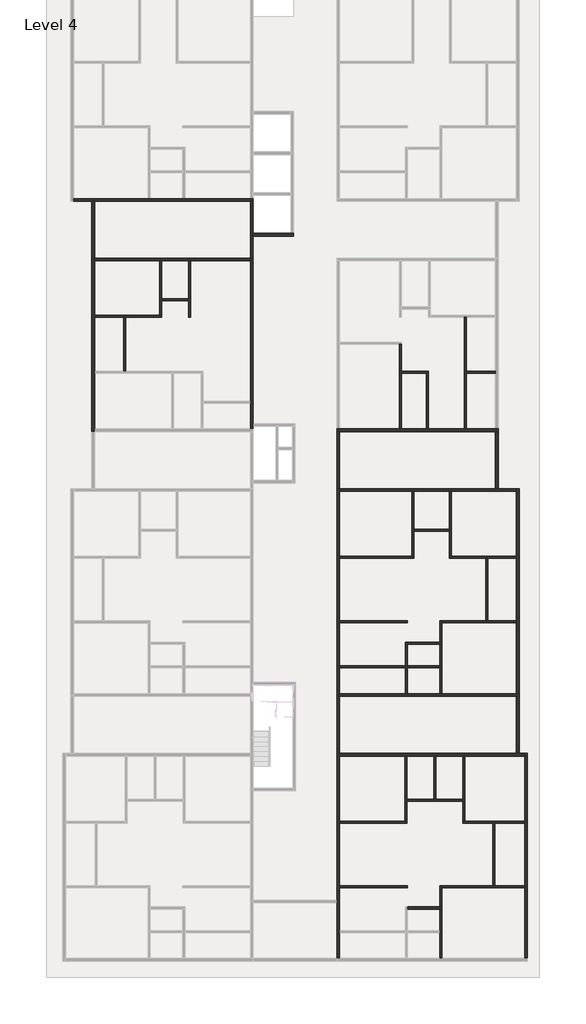
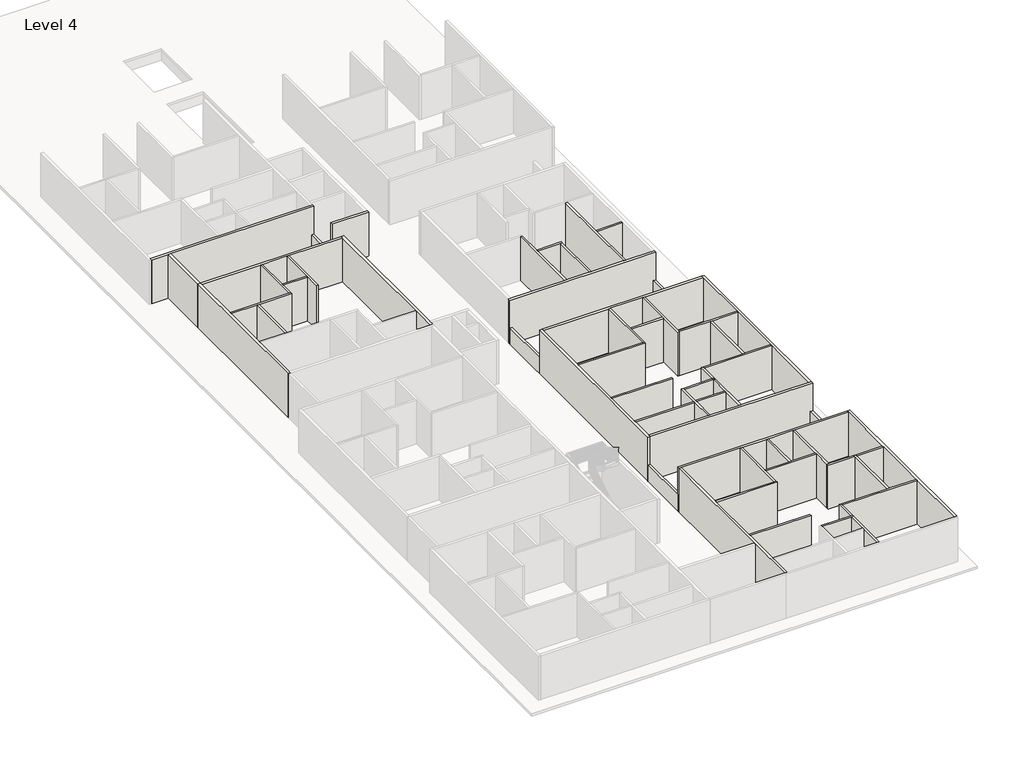
# One storey, part 2 of 8: 56 walls.
"""IFC4 building model written with IfcOpenShell, lengths in millimetres."""

from ifc_helpers import new_model, si_unit, frame, origin, place, context, project, spatial, polyline, outline, extrude, faceted_brep, element, save

model = new_model("IFC4")

# Units and contexts
model_context = context("Model", 3, world=origin())
ifc_project = project(units=[si_unit("LENGTHUNIT", "METRE", prefix="MILLI")], contexts=[model_context])

# Site, building, storey
site = spatial("IfcSite", under=ifc_project)
building = spatial("IfcBuilding", under=site)
storey = spatial("IfcBuildingStorey", under=building, Name="Level 4", Elevation=34378.6172466)

# Walls
placement = place(None, origin())
element("IfcWall", 1, ObjectType="4.5\"", at=placement, inside=storey, context=model_context, shape_type="Brep", body=[
    faceted_brep([(-12531.5544854, 2100.0216096, 34378.6172466), (-10907.2415084, 2100.0216096, 34378.6172466), (-10792.9415084, 2100.0216096, 34378.6172466), (-8759.6544854, 2100.0216096, 34378.6172466), (-8759.6544854, 2100.0216096, 37426.6172466), (-10792.9415084, 2100.0216096, 37426.6172466), (-10907.2415084, 2100.0216096, 37426.6172466), (-12531.5544854, 2100.0216096, 37426.6172466), (-12531.5544854, 2214.3216096, 34378.6172466), (-12531.5544854, 2214.3216096, 37426.6172466), (-8873.9544854, 2214.3216096, 37426.6172466), (-8759.6544854, 2214.3216096, 37426.6172466), (-8759.6544854, 2214.3216096, 34378.6172466), (-8873.9544854, 2214.3216096, 34378.6172466)], [[[0, 1, 2, 3, 4, 5, 6, 7]], [[8, 9, 10, 11, 12, 13]], [[3, 2, 1, 0, 8, 13, 12]], [[0, 7, 9, 8]], [[4, 3, 12, 11]], [[7, 6, 5, 4, 11, 10, 9]]]),
])
element("IfcWall", 2, ObjectType="4.5\"", at=placement, inside=storey, context=model_context, shape_type="Brep", body=[
    faceted_brep([(-8759.6544854, 2214.3216096, 34378.6172466), (-8759.6544854, 3014.4216096, 34378.6172466), (-8759.6544854, 3128.7216096, 34378.6172466), (-8759.6544854, 5264.2743917, 34378.6172466), (-8759.6544854, 5264.2743917, 37426.6172466), (-8759.6544854, 3128.7216096, 37426.6172466), (-8759.6544854, 3014.4216096, 37426.6172466), (-8759.6544854, 2214.3216096, 37426.6172466), (-8873.9544854, 2214.3216096, 34378.6172466), (-8873.9544854, 2214.3216096, 37426.6172466), (-8873.9544854, 5264.2743917, 37426.6172466), (-8873.9544854, 5264.2743917, 34378.6172466)], [[[0, 1, 2, 3, 4, 5, 6, 7]], [[8, 9, 10, 11]], [[3, 2, 1, 0, 8, 11]], [[0, 7, 9, 8]], [[4, 3, 11, 10]], [[7, 6, 5, 4, 10, 9]]]),
])
element("IfcWall", 3, ObjectType="4.5\"", at=placement, inside=storey, context=model_context, shape_type="Brep", body=[
    faceted_brep([(-7235.6544854, 5264.2743917, 34378.6172466), (-7235.6544854, 3128.7216096, 34378.6172466), (-7235.6544854, 3014.4216096, 34378.6172466), (-7235.6544854, 2100.0216096, 34378.6172466), (-7235.6544854, 2100.0216096, 37426.6172466), (-7235.6544854, 3014.4216096, 37426.6172466), (-7235.6544854, 3128.7216096, 37426.6172466), (-7235.6544854, 5264.2743917, 37426.6172466), (-7121.3544854, 5264.2743917, 34378.6172466), (-7121.3544854, 5264.2743917, 37426.6172466), (-7121.3544854, 2100.0216096, 37426.6172466), (-7121.3544854, 2100.0216096, 34378.6172466)], [[[0, 1, 2, 3, 4, 5, 6, 7]], [[8, 9, 10, 11]], [[3, 2, 1, 0, 8, 11]], [[4, 3, 11, 10]], [[0, 7, 9, 8]], [[7, 6, 5, 4, 10, 9]]]),
])
element("IfcWall", 4, ObjectType="4.5\"", at=placement, inside=storey, context=model_context, shape_type="SweptSolid", body=[
    extrude(outline(polyline([(-7235.6544854, 3014.4216096), (-8759.6544854, 3014.4216096), (-8759.6544854, 3128.7216096), (-7235.6544854, 3128.7216096), (-7235.6544854, 3014.4216096)])), frame((0.0, 0.0, 34378.6172466), z_axis=(0.0, 0.0, 1.0), x_axis=(1.0, 0.0, 0.0)), (0.0, 0.0, 1.0), 3048.0),
])
element("IfcWall", 5, ObjectType="4.5\"", at=placement, inside=storey, context=model_context, shape_type="SweptSolid", body=[
    extrude(outline(polyline([(-10907.2415084, -947.4344126), (-10907.2415084, 2100.0216096), (-10792.9415084, 2100.0216096), (-10792.9415084, -947.4344126), (-10907.2415084, -947.4344126)])), frame((0.0, 0.0, 34378.6172466), z_axis=(0.0, 0.0, 1.0), x_axis=(1.0, 0.0, 0.0)), (0.0, 0.0, 1.0), 3048.0),
])
element("IfcWall", 6, ObjectType="4.5\"", at=placement, inside=storey, context=model_context, shape_type="Brep", body=[
    faceted_brep([(5056.6584916, -31173.4344126, 34378.6172466), (6885.4584916, -31173.4344126, 34378.6172466), (6999.7584916, -31173.4344126, 34378.6172466), (6999.7584916, -31173.4344126, 37426.6172466), (6885.4584916, -31173.4344126, 37426.6172466), (5056.6584916, -31173.4344126, 37426.6172466), (5056.6584916, -31059.1344126, 34378.6172466), (5056.6584916, -31059.1344126, 37426.6172466), (6885.4584916, -31059.1344126, 37426.6172466), (6999.7584916, -31059.1344126, 37426.6172466), (6999.7584916, -31059.1344126, 34378.6172466), (6885.4584916, -31059.1344126, 34378.6172466)], [[[0, 1, 2, 3, 4, 5]], [[6, 7, 8, 9, 10, 11]], [[2, 1, 0, 6, 11, 10]], [[0, 5, 7, 6]], [[3, 2, 10, 9]], [[5, 4, 3, 9, 8, 7]]]),
])
element("IfcWall", 7, ObjectType="4.5\"", at=placement, inside=storey, context=model_context, shape_type="Brep", body=[
    faceted_brep([(6885.4584916, -31173.4344126, 34378.6172466), (6885.4584916, -32392.6344126, 34378.6172466), (6885.4584916, -32506.9344126, 34378.6172466), (6885.4584916, -33954.7344126, 34378.6172466), (6885.4584916, -33954.7344126, 37426.6172466), (6885.4584916, -32506.9344126, 37426.6172466), (6885.4584916, -32392.6344126, 37426.6172466), (6885.4584916, -31173.4344126, 37426.6172466), (6999.7584916, -31173.4344126, 34378.6172466), (6999.7584916, -31173.4344126, 37426.6172466), (6999.7584916, -33954.7344126, 37426.6172466), (6999.7584916, -33954.7344126, 34378.6172466)], [[[0, 1, 2, 3, 4, 5, 6, 7]], [[8, 9, 10, 11]], [[3, 2, 1, 0, 8, 11]], [[0, 7, 9, 8]], [[4, 3, 11, 10]], [[7, 6, 5, 4, 10, 9]]]),
])
element("IfcWall", 8, ObjectType="4.5\"", at=placement, inside=storey, context=model_context, shape_type="Brep", body=[
    faceted_brep([(6999.7584916, -31059.1344126, 34378.6172466), (6999.7584916, -29966.9344126, 34378.6172466), (6999.7584916, -29852.6344126, 34378.6172466), (6999.7584916, -29852.6344126, 37426.6172466), (6999.7584916, -29966.9344126, 37426.6172466), (6999.7584916, -31059.1344126, 37426.6172466), (6885.4584916, -31059.1344126, 34378.6172466), (6885.4584916, -31059.1344126, 37426.6172466), (6885.4584916, -29852.6344126, 37426.6172466), (6885.4584916, -29852.6344126, 34378.6172466)], [[[0, 1, 2, 3, 4, 5]], [[6, 7, 8, 9]], [[2, 1, 0, 6, 9]], [[0, 5, 7, 6]], [[3, 2, 9, 8]], [[5, 4, 3, 8, 7]]]),
])
element("IfcWall", 9, ObjectType="4.5\"", at=placement, inside=storey, context=model_context, shape_type="Brep", body=[
    faceted_brep([(6999.7584916, -29966.9344126, 34378.6172466), (11660.6584916, -29966.9344126, 34378.6172466), (11660.6584916, -29966.9344126, 37426.6172466), (6999.7584916, -29966.9344126, 37426.6172466), (6999.7584916, -29852.6344126, 34378.6172466), (6999.7584916, -29852.6344126, 37426.6172466), (9869.9584916, -29852.6344126, 37426.6172466), (9984.2584916, -29852.6344126, 37426.6172466), (11660.6584916, -29852.6344126, 37426.6172466), (11660.6584916, -29852.6344126, 34378.6172466), (9984.2584916, -29852.6344126, 34378.6172466), (9869.9584916, -29852.6344126, 34378.6172466)], [[[0, 1, 2, 3]], [[4, 5, 6, 7, 8, 9, 10, 11]], [[1, 0, 4, 11, 10, 9]], [[0, 3, 5, 4]], [[2, 1, 9, 8]], [[3, 2, 8, 7, 6, 5]]]),
])
element("IfcWall", 10, ObjectType="4.5\"", at=placement, inside=storey, context=model_context, shape_type="SweptSolid", body=[
    extrude(outline(polyline([(5056.6584916, -29966.9344126), (1259.3584916, -29966.9344126), (1259.3584916, -29852.6344126), (5056.6584916, -29852.6344126), (5056.6584916, -29966.9344126)])), frame((0.0, 0.0, 34378.6172466), z_axis=(0.0, 0.0, 1.0), x_axis=(1.0, 0.0, 0.0)), (0.0, 0.0, 1.0), 3048.0),
])
element("IfcWall", 11, ObjectType="4.5\"", at=placement, inside=storey, context=model_context, shape_type="Brep", body=[
    faceted_brep([(1259.3584916, -26347.4344126, 34378.6172466), (5031.2584916, -26347.4344126, 34378.6172466), (5031.2584916, -26347.4344126, 37426.6172466), (1259.3584916, -26347.4344126, 37426.6172466), (1259.3584916, -26233.1344126, 34378.6172466), (1259.3584916, -26233.1344126, 37426.6172466), (4916.9584916, -26233.1344126, 37426.6172466), (5031.2584916, -26233.1344126, 37426.6172466), (5031.2584916, -26233.1344126, 34378.6172466), (4916.9584916, -26233.1344126, 34378.6172466)], [[[0, 1, 2, 3]], [[4, 5, 6, 7, 8, 9]], [[1, 0, 4, 9, 8]], [[0, 3, 5, 4]], [[2, 1, 8, 7]], [[3, 2, 7, 6, 5]]]),
])
element("IfcWall", 12, ObjectType="4.5\"", at=placement, inside=storey, context=model_context, shape_type="Brep", body=[
    faceted_brep([(5031.2584916, -26233.1344126, 34378.6172466), (5031.2584916, -25128.2344126, 34378.6172466), (5031.2584916, -25013.9344126, 34378.6172466), (5031.2584916, -22575.5344126, 34378.6172466), (5031.2584916, -22575.5344126, 37426.6172466), (5031.2584916, -25013.9344126, 37426.6172466), (5031.2584916, -25128.2344126, 37426.6172466), (5031.2584916, -26233.1344126, 37426.6172466), (4916.9584916, -26233.1344126, 34378.6172466), (4916.9584916, -26233.1344126, 37426.6172466), (4916.9584916, -22575.5344126, 37426.6172466), (4916.9584916, -22575.5344126, 34378.6172466)], [[[0, 1, 2, 3, 4, 5, 6, 7]], [[8, 9, 10, 11]], [[3, 2, 1, 0, 8, 11]], [[0, 7, 9, 8]], [[4, 3, 11, 10]], [[7, 6, 5, 4, 10, 9]]]),
])
element("IfcWall", 13, ObjectType="4.5\"", at=placement, inside=storey, context=model_context, shape_type="Brep", body=[
    faceted_brep([(9984.2584916, -29852.6344126, 34378.6172466), (9984.2584916, -26347.4344126, 34378.6172466), (9984.2584916, -26233.1344126, 34378.6172466), (9984.2584916, -26233.1344126, 37426.6172466), (9984.2584916, -26347.4344126, 37426.6172466), (9984.2584916, -29852.6344126, 37426.6172466), (9869.9584916, -29852.6344126, 34378.6172466), (9869.9584916, -29852.6344126, 37426.6172466), (9869.9584916, -26347.4344126, 37426.6172466), (9869.9584916, -26233.1344126, 37426.6172466), (9869.9584916, -26233.1344126, 34378.6172466), (9869.9584916, -26347.4344126, 34378.6172466)], [[[0, 1, 2, 3, 4, 5]], [[6, 7, 8, 9, 10, 11]], [[2, 1, 0, 6, 11, 10]], [[0, 5, 7, 6]], [[3, 2, 10, 9]], [[5, 4, 3, 9, 8, 7]]]),
])
element("IfcWall", 14, ObjectType="4.5\"", at=placement, inside=storey, context=model_context, shape_type="SweptSolid", body=[
    extrude(outline(polyline([(11660.6584916, -26347.4344126), (9984.2584916, -26347.4344126), (9984.2584916, -26233.1344126), (11660.6584916, -26233.1344126), (11660.6584916, -26347.4344126)])), frame((0.0, 0.0, 34378.6172466), z_axis=(0.0, 0.0, 1.0), x_axis=(1.0, 0.0, 0.0)), (0.0, 0.0, 1.0), 3048.0),
])
element("IfcWall", 15, ObjectType="4.5\"", at=placement, inside=storey, context=model_context, shape_type="Brep", body=[
    faceted_brep([(9869.9584916, -26233.1344126, 34378.6172466), (8307.8584916, -26233.1344126, 34378.6172466), (8193.5584916, -26233.1344126, 34378.6172466), (8193.5584916, -26233.1344126, 37426.6172466), (8307.8584916, -26233.1344126, 37426.6172466), (9869.9584916, -26233.1344126, 37426.6172466), (9869.9584916, -26347.4344126, 34378.6172466), (9869.9584916, -26347.4344126, 37426.6172466), (8193.5584916, -26347.4344126, 37426.6172466), (8193.5584916, -26347.4344126, 34378.6172466)], [[[0, 1, 2, 3, 4, 5]], [[6, 7, 8, 9]], [[2, 1, 0, 6, 9]], [[0, 5, 7, 6]], [[3, 2, 9, 8]], [[5, 4, 3, 8, 7]]]),
])
element("IfcWall", 16, ObjectType="4.5\"", at=placement, inside=storey, context=model_context, shape_type="Brep", body=[
    faceted_brep([(8307.8584916, -26233.1344126, 34378.6172466), (8307.8584916, -22575.5344126, 34378.6172466), (8307.8584916, -22575.5344126, 37426.6172466), (8307.8584916, -26233.1344126, 37426.6172466), (8193.5584916, -26233.1344126, 34378.6172466), (8193.5584916, -26233.1344126, 37426.6172466), (8193.5584916, -25128.2344126, 37426.6172466), (8193.5584916, -25013.9344126, 37426.6172466), (8193.5584916, -22575.5344126, 37426.6172466), (8193.5584916, -22575.5344126, 34378.6172466), (8193.5584916, -25013.9344126, 34378.6172466), (8193.5584916, -25128.2344126, 34378.6172466)], [[[0, 1, 2, 3]], [[4, 5, 6, 7, 8, 9, 10, 11]], [[1, 0, 4, 11, 10, 9]], [[0, 3, 5, 4]], [[2, 1, 9, 8]], [[3, 2, 8, 7, 6, 5]]]),
])
element("IfcWall", 17, ObjectType="4.5\"", at=placement, inside=storey, context=model_context, shape_type="Brep", body=[
    faceted_brep([(5031.2584916, -25128.2344126, 34378.6172466), (8193.5584916, -25128.2344126, 34378.6172466), (8193.5584916, -25128.2344126, 37426.6172466), (5031.2584916, -25128.2344126, 37426.6172466), (5031.2584916, -25013.9344126, 34378.6172466), (5031.2584916, -25013.9344126, 37426.6172466), (6555.2584916, -25013.9344126, 37426.6172466), (6669.5584916, -25013.9344126, 37426.6172466), (8193.5584916, -25013.9344126, 37426.6172466), (8193.5584916, -25013.9344126, 34378.6172466), (6669.5584916, -25013.9344126, 34378.6172466), (6555.2584916, -25013.9344126, 34378.6172466)], [[[0, 1, 2, 3]], [[4, 5, 6, 7, 8, 9, 10, 11]], [[1, 0, 4, 11, 10, 9]], [[0, 3, 5, 4]], [[2, 1, 9, 8]], [[3, 2, 8, 7, 6, 5]]]),
])
element("IfcWall", 18, ObjectType="4.5\"", at=placement, inside=storey, context=model_context, shape_type="SweptSolid", body=[
    extrude(outline(polyline([(6555.2584916, -25013.9344126), (6555.2584916, -22575.5344126), (6669.5584916, -22575.5344126), (6669.5584916, -25013.9344126), (6555.2584916, -25013.9344126)])), frame((0.0, 0.0, 34378.6172466), z_axis=(0.0, 0.0, 1.0), x_axis=(1.0, 0.0, 0.0)), (0.0, 0.0, 1.0), 3048.0),
])
element("IfcWall", 19, ObjectType="4.5\"", at=placement, inside=storey, context=model_context, shape_type="SweptSolid", body=[
    extrude(outline(polyline([(4942.3584916, -17622.5344126), (1259.3584916, -17622.5344126), (1259.3584916, -17508.2344126), (4942.3584916, -17508.2344126), (4942.3584916, -17622.5344126)])), frame((0.0, 0.0, 34378.6172466), z_axis=(0.0, 0.0, 1.0), x_axis=(1.0, 0.0, 0.0)), (0.0, 0.0, 1.0), 3048.0),
])
element("IfcWall", 20, ObjectType="4.5\"", at=placement, inside=storey, context=model_context, shape_type="Brep", body=[
    faceted_brep([(4942.3584916, -16174.7344126, 34378.6172466), (4942.3584916, -17508.2344126, 34378.6172466), (4942.3584916, -17622.5344126, 34378.6172466), (4942.3584916, -19070.3344126, 34378.6172466), (4942.3584916, -19070.3344126, 37426.6172466), (4942.3584916, -17622.5344126, 37426.6172466), (4942.3584916, -17508.2344126, 37426.6172466), (4942.3584916, -16174.7344126, 37426.6172466), (5056.6584916, -16174.7344126, 34378.6172466), (5056.6584916, -16174.7344126, 37426.6172466), (5056.6584916, -16289.0344126, 37426.6172466), (5056.6584916, -17508.2344126, 37426.6172466), (5056.6584916, -17622.5344126, 37426.6172466), (5056.6584916, -19070.3344126, 37426.6172466), (5056.6584916, -19070.3344126, 34378.6172466), (5056.6584916, -17622.5344126, 34378.6172466), (5056.6584916, -17508.2344126, 34378.6172466), (5056.6584916, -16289.0344126, 34378.6172466)], [[[0, 1, 2, 3, 4, 5, 6, 7]], [[8, 9, 10, 11, 12, 13, 14, 15, 16, 17]], [[3, 2, 1, 0, 8, 17, 16, 15, 14]], [[4, 3, 14, 13]], [[0, 7, 9, 8]], [[7, 6, 5, 4, 13, 12, 11, 10, 9]]]),
])
element("IfcWall", 21, ObjectType="4.5\"", at=placement, inside=storey, context=model_context, shape_type="Brep", body=[
    faceted_brep([(5056.6584916, -16289.0344126, 34378.6172466), (6885.4584916, -16289.0344126, 34378.6172466), (6999.7584916, -16289.0344126, 34378.6172466), (6999.7584916, -16289.0344126, 37426.6172466), (6885.4584916, -16289.0344126, 37426.6172466), (5056.6584916, -16289.0344126, 37426.6172466), (5056.6584916, -16174.7344126, 34378.6172466), (5056.6584916, -16174.7344126, 37426.6172466), (6885.4584916, -16174.7344126, 37426.6172466), (6999.7584916, -16174.7344126, 37426.6172466), (6999.7584916, -16174.7344126, 34378.6172466), (6885.4584916, -16174.7344126, 34378.6172466)], [[[0, 1, 2, 3, 4, 5]], [[6, 7, 8, 9, 10, 11]], [[2, 1, 0, 6, 11, 10]], [[0, 5, 7, 6]], [[3, 2, 10, 9]], [[5, 4, 3, 9, 8, 7]]]),
])
element("IfcWall", 22, ObjectType="4.5\"", at=placement, inside=storey, context=model_context, shape_type="Brep", body=[
    faceted_brep([(6885.4584916, -16289.0344126, 34378.6172466), (6885.4584916, -17508.2344126, 34378.6172466), (6885.4584916, -17622.5344126, 34378.6172466), (6885.4584916, -19070.3344126, 34378.6172466), (6885.4584916, -19070.3344126, 37426.6172466), (6885.4584916, -17622.5344126, 37426.6172466), (6885.4584916, -17508.2344126, 37426.6172466), (6885.4584916, -16289.0344126, 37426.6172466), (6999.7584916, -16289.0344126, 34378.6172466), (6999.7584916, -16289.0344126, 37426.6172466), (6999.7584916, -19070.3344126, 37426.6172466), (6999.7584916, -19070.3344126, 34378.6172466)], [[[0, 1, 2, 3, 4, 5, 6, 7]], [[8, 9, 10, 11]], [[3, 2, 1, 0, 8, 11]], [[0, 7, 9, 8]], [[4, 3, 11, 10]], [[7, 6, 5, 4, 10, 9]]]),
])
element("IfcWall", 23, ObjectType="4.5\"", at=placement, inside=storey, context=model_context, shape_type="SweptSolid", body=[
    extrude(outline(polyline([(6885.4584916, -17622.5344126), (5056.6584916, -17622.5344126), (5056.6584916, -17508.2344126), (6885.4584916, -17508.2344126), (6885.4584916, -17622.5344126)])), frame((0.0, 0.0, 34378.6172466), z_axis=(0.0, 0.0, 1.0), x_axis=(1.0, 0.0, 0.0)), (0.0, 0.0, 1.0), 3048.0),
])
element("IfcWall", 24, ObjectType="4.5\"", at=placement, inside=storey, context=model_context, shape_type="Brep", body=[
    faceted_brep([(6999.7584916, -16174.7344126, 34378.6172466), (6999.7584916, -15082.5344126, 34378.6172466), (6999.7584916, -14968.2344126, 34378.6172466), (6999.7584916, -14968.2344126, 37426.6172466), (6999.7584916, -15082.5344126, 37426.6172466), (6999.7584916, -16174.7344126, 37426.6172466), (6885.4584916, -16174.7344126, 34378.6172466), (6885.4584916, -16174.7344126, 37426.6172466), (6885.4584916, -14968.2344126, 37426.6172466), (6885.4584916, -14968.2344126, 34378.6172466)], [[[0, 1, 2, 3, 4, 5]], [[6, 7, 8, 9]], [[2, 1, 0, 6, 9]], [[0, 5, 7, 6]], [[3, 2, 9, 8]], [[5, 4, 3, 8, 7]]]),
])
element("IfcWall", 25, ObjectType="4.5\"", at=placement, inside=storey, context=model_context, shape_type="Brep", body=[
    faceted_brep([(6999.7584916, -15082.5344126, 34378.6172466), (11208.5214687, -15082.5344126, 34378.6172466), (11208.5214687, -15082.5344126, 37426.6172466), (6999.7584916, -15082.5344126, 37426.6172466), (6999.7584916, -14968.2344126, 34378.6172466), (6999.7584916, -14968.2344126, 37426.6172466), (9469.9084916, -14968.2344126, 37426.6172466), (9584.2084916, -14968.2344126, 37426.6172466), (11208.5214687, -14968.2344126, 37426.6172466), (11208.5214687, -14968.2344126, 34378.6172466), (9584.2084916, -14968.2344126, 34378.6172466), (9469.9084916, -14968.2344126, 34378.6172466)], [[[0, 1, 2, 3]], [[4, 5, 6, 7, 8, 9, 10, 11]], [[1, 0, 4, 11, 10, 9]], [[0, 3, 5, 4]], [[2, 1, 9, 8]], [[3, 2, 8, 7, 6, 5]]]),
])
element("IfcWall", 26, ObjectType="4.5\"", at=placement, inside=storey, context=model_context, shape_type="SweptSolid", body=[
    extrude(outline(polyline([(5056.6584916, -15082.5344126), (1259.3584916, -15082.5344126), (1259.3584916, -14968.2344126), (5056.6584916, -14968.2344126), (5056.6584916, -15082.5344126)])), frame((0.0, 0.0, 34378.6172466), z_axis=(0.0, 0.0, 1.0), x_axis=(1.0, 0.0, 0.0)), (0.0, 0.0, 1.0), 3048.0),
])
element("IfcWall", 27, ObjectType="4.5\"", at=placement, inside=storey, context=model_context, shape_type="Brep", body=[
    faceted_brep([(1259.3584916, -11463.0344126, 34378.6172466), (5430.0214687, -11463.0344126, 34378.6172466), (5430.0214687, -11463.0344126, 37426.6172466), (1259.3584916, -11463.0344126, 37426.6172466), (1259.3584916, -11348.7344126, 34378.6172466), (1259.3584916, -11348.7344126, 37426.6172466), (5315.7214687, -11348.7344126, 37426.6172466), (5430.0214687, -11348.7344126, 37426.6172466), (5430.0214687, -11348.7344126, 34378.6172466), (5315.7214687, -11348.7344126, 34378.6172466)], [[[0, 1, 2, 3]], [[4, 5, 6, 7, 8, 9]], [[1, 0, 4, 9, 8]], [[0, 3, 5, 4]], [[2, 1, 8, 7]], [[3, 2, 7, 6, 5]]]),
])
element("IfcWall", 28, ObjectType="4.5\"", at=placement, inside=storey, context=model_context, shape_type="Brep", body=[
    faceted_brep([(5430.0214687, -11348.7344126, 34378.6172466), (5430.0214687, -9939.0344126, 34378.6172466), (5430.0214687, -9824.7344126, 34378.6172466), (5430.0214687, -7691.1344126, 34378.6172466), (5430.0214687, -7691.1344126, 37426.6172466), (5430.0214687, -9824.7344126, 37426.6172466), (5430.0214687, -9939.0344126, 37426.6172466), (5430.0214687, -11348.7344126, 37426.6172466), (5315.7214687, -11348.7344126, 34378.6172466), (5315.7214687, -11348.7344126, 37426.6172466), (5315.7214687, -7691.1344126, 37426.6172466), (5315.7214687, -7691.1344126, 34378.6172466)], [[[0, 1, 2, 3, 4, 5, 6, 7]], [[8, 9, 10, 11]], [[3, 2, 1, 0, 8, 11]], [[0, 7, 9, 8]], [[4, 3, 11, 10]], [[7, 6, 5, 4, 10, 9]]]),
])
element("IfcWall", 29, ObjectType="4.5\"", at=placement, inside=storey, context=model_context, shape_type="SweptSolid", body=[
    extrude(outline(polyline([(7436.6214687, -9939.0344126), (5430.0214687, -9939.0344126), (5430.0214687, -9824.7344126), (7436.6214687, -9824.7344126), (7436.6214687, -9939.0344126)])), frame((0.0, 0.0, 34378.6172466), z_axis=(0.0, 0.0, 1.0), x_axis=(1.0, 0.0, 0.0)), (0.0, 0.0, 1.0), 3048.0),
])
element("IfcWall", 30, ObjectType="4.5\"", at=placement, inside=storey, context=model_context, shape_type="Brep", body=[
    faceted_brep([(7436.6214687, -7691.1344126, 34378.6172466), (7436.6214687, -9824.7344126, 34378.6172466), (7436.6214687, -9939.0344126, 34378.6172466), (7436.6214687, -11463.0344126, 34378.6172466), (7436.6214687, -11463.0344126, 37426.6172466), (7436.6214687, -9939.0344126, 37426.6172466), (7436.6214687, -9824.7344126, 37426.6172466), (7436.6214687, -7691.1344126, 37426.6172466), (7550.9214687, -7691.1344126, 34378.6172466), (7550.9214687, -7691.1344126, 37426.6172466), (7550.9214687, -11348.7344126, 37426.6172466), (7550.9214687, -11463.0344126, 37426.6172466), (7550.9214687, -11463.0344126, 34378.6172466), (7550.9214687, -11348.7344126, 34378.6172466)], [[[0, 1, 2, 3, 4, 5, 6, 7]], [[8, 9, 10, 11, 12, 13]], [[3, 2, 1, 0, 8, 13, 12]], [[0, 7, 9, 8]], [[4, 3, 12, 11]], [[7, 6, 5, 4, 11, 10, 9]]]),
])
element("IfcWall", 31, ObjectType="4.5\"", at=placement, inside=storey, context=model_context, shape_type="Brep", body=[
    faceted_brep([(7550.9214687, -11463.0344126, 34378.6172466), (9469.9084916, -11463.0344126, 34378.6172466), (9584.2084916, -11463.0344126, 34378.6172466), (11208.5214687, -11463.0344126, 34378.6172466), (11208.5214687, -11463.0344126, 37426.6172466), (9584.2084916, -11463.0344126, 37426.6172466), (9469.9084916, -11463.0344126, 37426.6172466), (7550.9214687, -11463.0344126, 37426.6172466), (7550.9214687, -11348.7344126, 34378.6172466), (7550.9214687, -11348.7344126, 37426.6172466), (11208.5214687, -11348.7344126, 37426.6172466), (11208.5214687, -11348.7344126, 34378.6172466)], [[[0, 1, 2, 3, 4, 5, 6, 7]], [[8, 9, 10, 11]], [[3, 2, 1, 0, 8, 11]], [[0, 7, 9, 8]], [[4, 3, 11, 10]], [[7, 6, 5, 4, 10, 9]]]),
])
element("IfcWall", 32, ObjectType="4.5\"", at=placement, inside=storey, context=model_context, shape_type="SweptSolid", body=[
    extrude(outline(polyline([(9469.9084916, -14968.2344126), (9469.9084916, -11463.0344126), (9584.2084916, -11463.0344126), (9584.2084916, -14968.2344126), (9469.9084916, -14968.2344126)])), frame((0.0, 0.0, 34378.6172466), z_axis=(0.0, 0.0, 1.0), x_axis=(1.0, 0.0, 0.0)), (0.0, 0.0, 1.0), 3048.0),
])
element("IfcWall", 33, ObjectType="4.5\"", at=placement, inside=storey, context=model_context, shape_type="Brep", body=[
    faceted_brep([(4610.8714687, 572.7745083, 34378.6172466), (4610.8714687, -4185.9344126, 34378.6172466), (4610.8714687, -4185.9344126, 37426.6172466), (4610.8714687, 572.7745083, 37426.6172466), (4725.1714687, 572.7745083, 34378.6172466), (4725.1714687, 572.7745083, 37426.6172466), (4725.1714687, -947.4344126, 37426.6172466), (4725.1714687, -1061.7344126, 37426.6172466), (4725.1714687, -4185.9344126, 37426.6172466), (4725.1714687, -4185.9344126, 34378.6172466), (4725.1714687, -1061.7344126, 34378.6172466), (4725.1714687, -947.4344126, 34378.6172466)], [[[0, 1, 2, 3]], [[4, 5, 6, 7, 8, 9, 10, 11]], [[1, 0, 4, 11, 10, 9]], [[0, 3, 5, 4]], [[2, 1, 9, 8]], [[3, 2, 8, 7, 6, 5]]]),
])
element("IfcWall", 34, ObjectType="4.5\"", at=placement, inside=storey, context=model_context, shape_type="Brep", body=[
    faceted_brep([(4725.1714687, -1061.7344126, 34378.6172466), (6134.8714687, -1061.7344126, 34378.6172466), (6249.1714687, -1061.7344126, 34378.6172466), (6249.1714687, -1061.7344126, 37426.6172466), (6134.8714687, -1061.7344126, 37426.6172466), (4725.1714687, -1061.7344126, 37426.6172466), (4725.1714687, -947.4344126, 34378.6172466), (4725.1714687, -947.4344126, 37426.6172466), (6249.1714687, -947.4344126, 37426.6172466), (6249.1714687, -947.4344126, 34378.6172466)], [[[0, 1, 2, 3, 4, 5]], [[6, 7, 8, 9]], [[2, 1, 0, 6, 9]], [[0, 5, 7, 6]], [[3, 2, 9, 8]], [[5, 4, 3, 8, 7]]]),
])
element("IfcWall", 35, ObjectType="4.5\"", at=placement, inside=storey, context=model_context, shape_type="SweptSolid", body=[
    extrude(outline(polyline([(6134.8714687, -4185.9344126), (6134.8714687, -1061.7344126), (6249.1714687, -1061.7344126), (6249.1714687, -4185.9344126), (6134.8714687, -4185.9344126)])), frame((0.0, 0.0, 34378.6172466), z_axis=(0.0, 0.0, 1.0), x_axis=(1.0, 0.0, 0.0)), (0.0, 0.0, 1.0), 3048.0),
])
element("IfcWall", 36, ObjectType="4.5\"", at=placement, inside=storey, context=model_context, shape_type="Brep", body=[
    faceted_brep([(8396.7584916, -4185.9344126, 34378.6172466), (8396.7584916, -1061.7344126, 34378.6172466), (8396.7584916, -947.4344126, 34378.6172466), (8396.7584916, 2100.0216096, 34378.6172466), (8396.7584916, 2100.0216096, 37426.6172466), (8396.7584916, -947.4344126, 37426.6172466), (8396.7584916, -1061.7344126, 37426.6172466), (8396.7584916, -4185.9344126, 37426.6172466), (8282.4584916, -4185.9344126, 34378.6172466), (8282.4584916, -4185.9344126, 37426.6172466), (8282.4584916, 2100.0216096, 37426.6172466), (8282.4584916, 2100.0216096, 34378.6172466)], [[[0, 1, 2, 3, 4, 5, 6, 7]], [[8, 9, 10, 11]], [[3, 2, 1, 0, 8, 11]], [[0, 7, 9, 8]], [[4, 3, 11, 10]], [[7, 6, 5, 4, 10, 9]]]),
])
element("IfcWall", 37, ObjectType="4.5\"", at=placement, inside=storey, context=model_context, shape_type="SweptSolid", body=[
    extrude(outline(polyline([(8396.7584916, -947.4344126), (10021.0714687, -947.4344126), (10021.0714687, -1061.7344126), (8396.7584916, -1061.7344126), (8396.7584916, -947.4344126)])), frame((0.0, 0.0, 34378.6172466), z_axis=(0.0, 0.0, 1.0), x_axis=(1.0, 0.0, 0.0)), (0.0, 0.0, 1.0), 3048.0),
])
element("IfcWall", 38, ObjectType="6\"", at=placement, inside=storey, context=model_context, shape_type="Brep", body=[
    faceted_brep([(-13719.0044854, 8615.1216096, 34378.6172466), (-12683.9544854, 8615.1216096, 34378.6172466), (-12531.5544854, 8615.1216096, 34378.6172466), (-3769.8415084, 8615.1216096, 34378.6172466), (-3617.4415084, 8615.1216096, 34378.6172466), (-3617.4415084, 8615.1216096, 35597.8172466), (-3617.4415084, 8615.1216096, 37426.6172466), (-12531.5544854, 8615.1216096, 37426.6172466), (-12683.9544854, 8615.1216096, 37426.6172466), (-13719.0044854, 8615.1216096, 37426.6172466), (-13719.0044854, 8767.5216096, 34378.6172466), (-13719.0044854, 8767.5216096, 37426.6172466), (-9510.2415084, 8767.5216096, 37426.6172466), (-9395.9415084, 8767.5216096, 37426.6172466), (-7567.1415084, 8767.5216096, 37426.6172466), (-7452.8415084, 8767.5216096, 37426.6172466), (-3769.8415084, 8767.5216096, 37426.6172466), (-3617.4415084, 8767.5216096, 37426.6172466), (-3617.4415084, 8767.5216096, 34378.6172466), (-3769.8415084, 8767.5216096, 34378.6172466), (-7452.8415084, 8767.5216096, 34378.6172466), (-7567.1415084, 8767.5216096, 34378.6172466), (-9395.9415084, 8767.5216096, 34378.6172466), (-9510.2415084, 8767.5216096, 34378.6172466)], [[[0, 1, 2, 3, 4, 5, 6, 7, 8, 9]], [[10, 11, 12, 13, 14, 15, 16, 17, 18, 19, 20, 21, 22, 23]], [[4, 3, 2, 1, 0, 10, 23, 22, 21, 20, 19, 18]], [[0, 9, 11, 10]], [[4, 18, 17, 6, 5]], [[9, 8, 7, 6, 17, 16, 15, 14, 13, 12, 11]]]),
])
element("IfcWall", 39, ObjectType="6\"", at=placement, inside=storey, context=model_context, shape_type="Brep", body=[
    faceted_brep([(-12683.9544854, 5416.6743917, 34378.6172466), (-12683.9544854, -4338.3344126, 34378.6172466), (-12683.9544854, -4338.3344126, 37426.6172466), (-12683.9544854, 5416.6743917, 37426.6172466), (-12531.5544854, 5416.6743917, 34378.6172466), (-12531.5544854, 5416.6743917, 37426.6172466), (-12531.5544854, 5264.2743917, 37426.6172466), (-12531.5544854, 2214.3216096, 37426.6172466), (-12531.5544854, 2100.0216096, 37426.6172466), (-12531.5544854, -947.4344126, 37426.6172466), (-12531.5544854, -1061.7344126, 37426.6172466), (-12531.5544854, -4185.9344126, 37426.6172466), (-12531.5544854, -4338.3344126, 37426.6172466), (-12531.5544854, -4338.3344126, 34378.6172466), (-12531.5544854, -4185.9344126, 34378.6172466), (-12531.5544854, -1061.7344126, 34378.6172466), (-12531.5544854, -947.4344126, 34378.6172466), (-12531.5544854, 2100.0216096, 34378.6172466), (-12531.5544854, 2214.3216096, 34378.6172466), (-12531.5544854, 5264.2743917, 34378.6172466)], [[[0, 1, 2, 3]], [[4, 5, 6, 7, 8, 9, 10, 11, 12, 13, 14, 15, 16, 17, 18, 19]], [[1, 0, 4, 19, 18, 17, 16, 15, 14, 13]], [[2, 1, 13, 12]], [[0, 3, 5, 4]], [[3, 2, 12, 11, 10, 9, 8, 7, 6, 5]]]),
])
element("IfcWall", 40, ObjectType="6\"", at=placement, inside=storey, context=model_context, shape_type="Brep", body=[
    faceted_brep([(-3617.4415084, -4185.9344126, 34378.6172466), (-3617.4415084, -4034.6751812, 34378.6172466), (-3617.4415084, -3882.2751812, 34378.6172466), (-3617.4415084, 5416.6743917, 34378.6172466), (-3617.4415084, 5416.6743917, 37426.6172466), (-3617.4415084, -3882.2751812, 37426.6172466), (-3617.4415084, -4034.6751812, 37426.6172466), (-3617.4415084, -4185.9344126, 37426.6172466), (-3769.8415084, -4185.9344126, 34378.6172466), (-3769.8415084, -4185.9344126, 37426.6172466), (-3769.8415084, -2738.1344126, 37426.6172466), (-3769.8415084, -2623.8344126, 37426.6172466), (-3769.8415084, 5264.2743917, 37426.6172466), (-3769.8415084, 5416.6743917, 37426.6172466), (-3769.8415084, 5416.6743917, 34378.6172466), (-3769.8415084, 5264.2743917, 34378.6172466), (-3769.8415084, -2623.8344126, 34378.6172466), (-3769.8415084, -2738.1344126, 34378.6172466)], [[[0, 1, 2, 3, 4, 5, 6, 7]], [[8, 9, 10, 11, 12, 13, 14, 15, 16, 17]], [[3, 2, 1, 0, 8, 17, 16, 15, 14]], [[0, 7, 9, 8]], [[3, 14, 13, 4]], [[7, 6, 5, 4, 13, 12, 11, 10, 9]]]),
])
element("IfcWall", 41, ObjectType="6\"", at=placement, inside=storey, context=model_context, shape_type="Brep", body=[
    faceted_brep([(-3769.8415084, 5416.6743917, 37426.6172466), (-3769.8415084, 5416.6743917, 34378.6172466), (-12531.5544854, 5416.6743917, 34378.6172466), (-12531.5544854, 5416.6743917, 37426.6172466), (-3769.8415084, 5264.2743917, 34378.6172466), (-3769.8415084, 5264.2743917, 37426.6172466), (-7121.3544854, 5264.2743917, 37426.6172466), (-7235.6544854, 5264.2743917, 37426.6172466), (-8759.6544854, 5264.2743917, 37426.6172466), (-8873.9544854, 5264.2743917, 37426.6172466), (-12531.5544854, 5264.2743917, 37426.6172466), (-12531.5544854, 5264.2743917, 34378.6172466), (-8873.9544854, 5264.2743917, 34378.6172466), (-8759.6544854, 5264.2743917, 34378.6172466), (-7235.6544854, 5264.2743917, 34378.6172466), (-7121.3544854, 5264.2743917, 34378.6172466)], [[[0, 1, 2, 3]], [[4, 5, 6, 7, 8, 9, 10, 11, 12, 13, 14, 15]], [[2, 1, 4, 15, 14, 13, 12, 11]], [[3, 2, 11, 10]], [[0, 5, 4, 1]], [[0, 3, 10, 9, 8, 7, 6, 5]]]),
])
element("IfcWall", 42, ObjectType="6\"", at=placement, inside=storey, context=model_context, shape_type="Brep", body=[
    faceted_brep([(11813.0584916, -33954.7344126, 34378.6172466), (11813.0584916, -22423.1344126, 34378.6172466), (11813.0584916, -22423.1344126, 37426.6172466), (11813.0584916, -33954.7344126, 37426.6172466), (11660.6584916, -33954.7344126, 34378.6172466), (11660.6584916, -33954.7344126, 37426.6172466), (11660.6584916, -29966.9344126, 37426.6172466), (11660.6584916, -29852.6344126, 37426.6172466), (11660.6584916, -26347.4344126, 37426.6172466), (11660.6584916, -26233.1344126, 37426.6172466), (11660.6584916, -22575.5344126, 37426.6172466), (11660.6584916, -22423.1344126, 37426.6172466), (11660.6584916, -22423.1344126, 34378.6172466), (11660.6584916, -22575.5344126, 34378.6172466), (11660.6584916, -26233.1344126, 34378.6172466), (11660.6584916, -26347.4344126, 34378.6172466), (11660.6584916, -29852.6344126, 34378.6172466), (11660.6584916, -29966.9344126, 34378.6172466)], [[[0, 1, 2, 3]], [[4, 5, 6, 7, 8, 9, 10, 11, 12, 13, 14, 15, 16, 17]], [[1, 0, 4, 17, 16, 15, 14, 13, 12]], [[0, 3, 5, 4]], [[2, 1, 12, 11]], [[3, 2, 11, 10, 9, 8, 7, 6, 5]]]),
])
element("IfcWall", 43, ObjectType="6\"", at=placement, inside=storey, context=model_context, shape_type="Brep", body=[
    faceted_brep([(11660.6584916, -22423.1344126, 34378.6172466), (11360.9214687, -22423.1344126, 34378.6172466), (11208.5214687, -22423.1344126, 34378.6172466), (1259.3584916, -22423.1344126, 34378.6172466), (1106.9584916, -22423.1344126, 34378.6172466), (1106.9584916, -22423.1344126, 35597.8172466), (1106.9584916, -22423.1344126, 37426.6172466), (11660.6584916, -22423.1344126, 37426.6172466), (11660.6584916, -22575.5344126, 34378.6172466), (11660.6584916, -22575.5344126, 37426.6172466), (8307.8584916, -22575.5344126, 37426.6172466), (8193.5584916, -22575.5344126, 37426.6172466), (6669.5584916, -22575.5344126, 37426.6172466), (6555.2584916, -22575.5344126, 37426.6172466), (5031.2584916, -22575.5344126, 37426.6172466), (4916.9584916, -22575.5344126, 37426.6172466), (1259.3584916, -22575.5344126, 37426.6172466), (1106.9584916, -22575.5344126, 37426.6172466), (1106.9584916, -22575.5344126, 34378.6172466), (1259.3584916, -22575.5344126, 34378.6172466), (4916.9584916, -22575.5344126, 34378.6172466), (5031.2584916, -22575.5344126, 34378.6172466), (6555.2584916, -22575.5344126, 34378.6172466), (6669.5584916, -22575.5344126, 34378.6172466), (8193.5584916, -22575.5344126, 34378.6172466), (8307.8584916, -22575.5344126, 34378.6172466)], [[[0, 1, 2, 3, 4, 5, 6, 7]], [[8, 9, 10, 11, 12, 13, 14, 15, 16, 17, 18, 19, 20, 21, 22, 23, 24, 25]], [[4, 3, 2, 1, 0, 8, 25, 24, 23, 22, 21, 20, 19, 18]], [[0, 7, 9, 8]], [[4, 18, 17, 6, 5]], [[7, 6, 17, 16, 15, 14, 13, 12, 11, 10, 9]]]),
])
element("IfcWall", 44, ObjectType="6\"", at=placement, inside=storey, context=model_context, shape_type="Brep", body=[
    faceted_brep([(1106.9584916, -22575.5344126, 37426.6172466), (1106.9584916, -22575.5344126, 34378.6172466), (1106.9584916, -30668.5325185, 34378.6172466), (1106.9584916, -30820.9325185, 34378.6172466), (1106.9584916, -33954.7344126, 34378.6172466), (1106.9584916, -33954.7344126, 37426.6172466), (1106.9584916, -30820.9325185, 37426.6172466), (1106.9584916, -30668.5325185, 37426.6172466), (1259.3584916, -22575.5344126, 34378.6172466), (1259.3584916, -22575.5344126, 37426.6172466), (1259.3584916, -26233.1344126, 37426.6172466), (1259.3584916, -26347.4344126, 37426.6172466), (1259.3584916, -29852.6344126, 37426.6172466), (1259.3584916, -29966.9344126, 37426.6172466), (1259.3584916, -32392.6344126, 37426.6172466), (1259.3584916, -32506.9344126, 37426.6172466), (1259.3584916, -33954.7344126, 37426.6172466), (1259.3584916, -33954.7344126, 34378.6172466), (1259.3584916, -32506.9344126, 34378.6172466), (1259.3584916, -32392.6344126, 34378.6172466), (1259.3584916, -29966.9344126, 34378.6172466), (1259.3584916, -29852.6344126, 34378.6172466), (1259.3584916, -26347.4344126, 34378.6172466), (1259.3584916, -26233.1344126, 34378.6172466)], [[[0, 1, 2, 3, 4, 5, 6, 7]], [[8, 9, 10, 11, 12, 13, 14, 15, 16, 17, 18, 19, 20, 21, 22, 23]], [[4, 3, 2, 1, 8, 23, 22, 21, 20, 19, 18, 17]], [[5, 4, 17, 16]], [[0, 9, 8, 1]], [[0, 7, 6, 5, 16, 15, 14, 13, 12, 11, 10, 9]]]),
])
element("IfcWall", 45, ObjectType="6\"", at=placement, inside=storey, context=model_context, shape_type="Brep", body=[
    faceted_brep([(1106.9584916, -7538.7344126, 37426.6172466), (1106.9584916, -7538.7344126, 34378.6172466), (1106.9584916, -19222.7344126, 34378.6172466), (1106.9584916, -19222.7344126, 37426.6172466), (1259.3584916, -7538.7344126, 34378.6172466), (1259.3584916, -7538.7344126, 37426.6172466), (1259.3584916, -7691.1344126, 37426.6172466), (1259.3584916, -11348.7344126, 37426.6172466), (1259.3584916, -11463.0344126, 37426.6172466), (1259.3584916, -14968.2344126, 37426.6172466), (1259.3584916, -15082.5344126, 37426.6172466), (1259.3584916, -17508.2344126, 37426.6172466), (1259.3584916, -17622.5344126, 37426.6172466), (1259.3584916, -19070.3344126, 37426.6172466), (1259.3584916, -19222.7344126, 37426.6172466), (1259.3584916, -19222.7344126, 34378.6172466), (1259.3584916, -19070.3344126, 34378.6172466), (1259.3584916, -17622.5344126, 34378.6172466), (1259.3584916, -17508.2344126, 34378.6172466), (1259.3584916, -15082.5344126, 34378.6172466), (1259.3584916, -14968.2344126, 34378.6172466), (1259.3584916, -11463.0344126, 34378.6172466), (1259.3584916, -11348.7344126, 34378.6172466), (1259.3584916, -7691.1344126, 34378.6172466)], [[[0, 1, 2, 3]], [[4, 5, 6, 7, 8, 9, 10, 11, 12, 13, 14, 15, 16, 17, 18, 19, 20, 21, 22, 23]], [[2, 1, 4, 23, 22, 21, 20, 19, 18, 17, 16, 15]], [[0, 5, 4, 1]], [[2, 15, 14, 3]], [[0, 3, 14, 13, 12, 11, 10, 9, 8, 7, 6, 5]]]),
])
element("IfcWall", 46, ObjectType="6\"", at=placement, inside=storey, context=model_context, shape_type="Brep", body=[
    faceted_brep([(1259.3584916, -19222.7344126, 37426.6172466), (1259.3584916, -19222.7344126, 34378.6172466), (11208.5214687, -19222.7344126, 34378.6172466), (11360.9214687, -19222.7344126, 34378.6172466), (11360.9214687, -19222.7344126, 35597.8172466), (11360.9214687, -19222.7344126, 37426.6172466), (1259.3584916, -19070.3344126, 34378.6172466), (1259.3584916, -19070.3344126, 37426.6172466), (4942.3584916, -19070.3344126, 37426.6172466), (5056.6584916, -19070.3344126, 37426.6172466), (6885.4584916, -19070.3344126, 37426.6172466), (6999.7584916, -19070.3344126, 37426.6172466), (11208.5214687, -19070.3344126, 37426.6172466), (11360.9214687, -19070.3344126, 37426.6172466), (11360.9214687, -19070.3344126, 34378.6172466), (11208.5214687, -19070.3344126, 34378.6172466), (6999.7584916, -19070.3344126, 34378.6172466), (6885.4584916, -19070.3344126, 34378.6172466), (5056.6584916, -19070.3344126, 34378.6172466), (4942.3584916, -19070.3344126, 34378.6172466)], [[[0, 1, 2, 3, 4, 5]], [[6, 7, 8, 9, 10, 11, 12, 13, 14, 15, 16, 17, 18, 19]], [[3, 2, 1, 6, 19, 18, 17, 16, 15, 14]], [[3, 14, 13, 5, 4]], [[0, 7, 6, 1]], [[0, 5, 13, 12, 11, 10, 9, 8, 7]]]),
])
element("IfcWall", 47, ObjectType="6\"", at=placement, inside=storey, context=model_context, shape_type="Brep", body=[
    faceted_brep([(11360.9214687, -19070.3344126, 37426.6172466), (11360.9214687, -19070.3344126, 34378.6172466), (11360.9214687, -7538.7344126, 34378.6172466), (11360.9214687, -7538.7344126, 37426.6172466), (11208.5214687, -19070.3344126, 34378.6172466), (11208.5214687, -19070.3344126, 37426.6172466), (11208.5214687, -15082.5344126, 37426.6172466), (11208.5214687, -14968.2344126, 37426.6172466), (11208.5214687, -11463.0344126, 37426.6172466), (11208.5214687, -11348.7344126, 37426.6172466), (11208.5214687, -7691.1344126, 37426.6172466), (11208.5214687, -7538.7344126, 37426.6172466), (11208.5214687, -7538.7344126, 34378.6172466), (11208.5214687, -7691.1344126, 34378.6172466), (11208.5214687, -11348.7344126, 34378.6172466), (11208.5214687, -11463.0344126, 34378.6172466), (11208.5214687, -14968.2344126, 34378.6172466), (11208.5214687, -15082.5344126, 34378.6172466)], [[[0, 1, 2, 3]], [[4, 5, 6, 7, 8, 9, 10, 11, 12, 13, 14, 15, 16, 17]], [[2, 1, 4, 17, 16, 15, 14, 13, 12]], [[3, 2, 12, 11]], [[0, 5, 4, 1]], [[0, 3, 11, 10, 9, 8, 7, 6, 5]]]),
])
element("IfcWall", 48, ObjectType="6\"", at=placement, inside=storey, context=model_context, shape_type="Brep", body=[
    faceted_brep([(11208.5214687, -7538.7344126, 34378.6172466), (10173.4714687, -7538.7344126, 34378.6172466), (10021.0714687, -7538.7344126, 34378.6172466), (1259.3584916, -7538.7344126, 34378.6172466), (1259.3584916, -7538.7344126, 37426.6172466), (11208.5214687, -7538.7344126, 37426.6172466), (11208.5214687, -7691.1344126, 34378.6172466), (11208.5214687, -7691.1344126, 37426.6172466), (7550.9214687, -7691.1344126, 37426.6172466), (7436.6214687, -7691.1344126, 37426.6172466), (5430.0214687, -7691.1344126, 37426.6172466), (5315.7214687, -7691.1344126, 37426.6172466), (1259.3584916, -7691.1344126, 37426.6172466), (1259.3584916, -7691.1344126, 34378.6172466), (5315.7214687, -7691.1344126, 34378.6172466), (5430.0214687, -7691.1344126, 34378.6172466), (7436.6214687, -7691.1344126, 34378.6172466), (7550.9214687, -7691.1344126, 34378.6172466)], [[[0, 1, 2, 3, 4, 5]], [[6, 7, 8, 9, 10, 11, 12, 13, 14, 15, 16, 17]], [[3, 2, 1, 0, 6, 17, 16, 15, 14, 13]], [[0, 5, 7, 6]], [[3, 13, 12, 4]], [[5, 4, 12, 11, 10, 9, 8, 7]]]),
])
element("IfcWall", 49, ObjectType="6\"", at=placement, inside=storey, context=model_context, shape_type="Brep", body=[
    faceted_brep([(1106.9584916, -4338.3344126, 37426.6172466), (1106.9584916, -4338.3344126, 35597.8172466), (1106.9584916, -4338.3344126, 34378.6172466), (1259.3584916, -4338.3344126, 34378.6172466), (10021.0714687, -4338.3344126, 34378.6172466), (10173.4714687, -4338.3344126, 34378.6172466), (10173.4714687, -4338.3344126, 35597.8172466), (10173.4714687, -4338.3344126, 37426.6172466), (1106.9584916, -4185.9344126, 34378.6172466), (1106.9584916, -4185.9344126, 37426.6172466), (1259.3584916, -4185.9344126, 37426.6172466), (4610.8714687, -4185.9344126, 37426.6172466), (4725.1714687, -4185.9344126, 37426.6172466), (6134.8714687, -4185.9344126, 37426.6172466), (6249.1714687, -4185.9344126, 37426.6172466), (8282.4584916, -4185.9344126, 37426.6172466), (8396.7584916, -4185.9344126, 37426.6172466), (10021.0714687, -4185.9344126, 37426.6172466), (10173.4714687, -4185.9344126, 37426.6172466), (10173.4714687, -4185.9344126, 34378.6172466), (10021.0714687, -4185.9344126, 34378.6172466), (8396.7584916, -4185.9344126, 34378.6172466), (8282.4584916, -4185.9344126, 34378.6172466), (6249.1714687, -4185.9344126, 34378.6172466), (6134.8714687, -4185.9344126, 34378.6172466), (4725.1714687, -4185.9344126, 34378.6172466), (4610.8714687, -4185.9344126, 34378.6172466), (1259.3584916, -4185.9344126, 34378.6172466)], [[[0, 1, 2, 3, 4, 5, 6, 7]], [[8, 9, 10, 11, 12, 13, 14, 15, 16, 17, 18, 19, 20, 21, 22, 23, 24, 25, 26, 27]], [[5, 4, 3, 2, 8, 27, 26, 25, 24, 23, 22, 21, 20, 19]], [[0, 9, 8, 2, 1]], [[5, 19, 18, 7, 6]], [[0, 7, 18, 17, 16, 15, 14, 13, 12, 11, 10, 9]]]),
])
element("IfcWall", 50, ObjectType="6\"", at=placement, inside=storey, context=model_context, shape_type="Brep", body=[
    faceted_brep([(-3617.4415084, 6659.2303368, 34378.6172466), (-1331.4415084, 6659.2303368, 34378.6172466), (-1331.4415084, 6659.2303368, 37426.6172466), (-3617.4415084, 6659.2303368, 37426.6172466), (-3617.4415084, 6811.6303368, 34378.6172466), (-3617.4415084, 6811.6303368, 37426.6172466), (-1483.8415084, 6811.6303368, 37426.6172466), (-1331.4415084, 6811.6303368, 37426.6172466), (-1331.4415084, 6811.6303368, 34378.6172466), (-1483.8415084, 6811.6303368, 34378.6172466)], [[[0, 1, 2, 3]], [[4, 5, 6, 7, 8, 9]], [[1, 0, 4, 9, 8]], [[3, 2, 7, 6, 5]], [[0, 3, 5, 4]], [[2, 1, 8, 7]]]),
])
element("IfcWall", 51, ObjectType="6\" 2", at=placement, inside=storey, context=model_context, shape_type="SweptSolid", body=[
    extrude(outline(polyline([(-12683.9544854, 5416.6743917), (-12683.9544854, 8615.1216096), (-12531.5544854, 8615.1216096), (-12531.5544854, 5416.6743917), (-12683.9544854, 5416.6743917)])), frame((0.0, 0.0, 34378.6172466), z_axis=(0.0, 0.0, 1.0), x_axis=(1.0, 0.0, 0.0)), (0.0, 0.0, 1.0), 3048.0),
])
element("IfcWall", 52, ObjectType="6\" 2", at=placement, inside=storey, context=model_context, shape_type="Brep", body=[
    faceted_brep([(-3769.8415084, 8615.1216096, 34378.6172466), (-3769.8415084, 5416.6743917, 34378.6172466), (-3769.8415084, 5416.6743917, 35597.8172466), (-3769.8415084, 8615.1216096, 35597.8172466), (-3617.4415084, 8615.1216096, 34378.6172466), (-3617.4415084, 8615.1216096, 35597.8172466), (-3617.4415084, 5416.6743917, 35597.8172466), (-3617.4415084, 5416.6743917, 34378.6172466), (-3617.4415084, 6659.2303368, 34378.6172466), (-3617.4415084, 6811.6303368, 34378.6172466)], [[[0, 1, 2, 3]], [[4, 5, 6, 7, 8, 9]], [[1, 0, 4, 9, 8, 7]], [[3, 2, 6, 5]], [[0, 3, 5, 4]], [[2, 1, 7, 6]]]),
])
element("IfcWall", 53, ObjectType="6\" 2", at=placement, inside=storey, context=model_context, shape_type="SweptSolid", body=[
    extrude(outline(polyline([(1106.9584916, -7538.7344126), (1106.9584916, -4338.3344126), (1259.3584916, -4338.3344126), (1259.3584916, -7538.7344126), (1106.9584916, -7538.7344126)])), frame((0.0, 0.0, 34378.6172466), z_axis=(0.0, 0.0, 1.0), x_axis=(1.0, 0.0, 0.0)), (0.0, 0.0, 1.0), 1219.2),
])
element("IfcWall", 54, ObjectType="6\" 2", at=placement, inside=storey, context=model_context, shape_type="SweptSolid", body=[
    extrude(outline(polyline([(10021.0714687, -7538.7344126), (10021.0714687, -4338.3344126), (10173.4714687, -4338.3344126), (10173.4714687, -7538.7344126), (10021.0714687, -7538.7344126)])), frame((0.0, 0.0, 34378.6172466), z_axis=(0.0, 0.0, 1.0), x_axis=(1.0, 0.0, 0.0)), (0.0, 0.0, 1.0), 1219.2),
])
element("IfcWall", 55, ObjectType="6\" 2", at=placement, inside=storey, context=model_context, shape_type="SweptSolid", body=[
    extrude(outline(polyline([(11208.5214687, -22423.1344126), (11208.5214687, -19222.7344126), (11360.9214687, -19222.7344126), (11360.9214687, -22423.1344126), (11208.5214687, -22423.1344126)])), frame((0.0, 0.0, 34378.6172466), z_axis=(0.0, 0.0, 1.0), x_axis=(1.0, 0.0, 0.0)), (0.0, 0.0, 1.0), 1219.2),
])
element("IfcWall", 56, ObjectType="6\" 2", at=placement, inside=storey, context=model_context, shape_type="SweptSolid", body=[
    extrude(outline(polyline([(1106.9584916, -22423.1344126), (1106.9584916, -19222.7344126), (1259.3584916, -19222.7344126), (1259.3584916, -22423.1344126), (1106.9584916, -22423.1344126)])), frame((0.0, 0.0, 34378.6172466), z_axis=(0.0, 0.0, 1.0), x_axis=(1.0, 0.0, 0.0)), (0.0, 0.0, 1.0), 1219.2),
])

save(model, "model.ifc")

# Revit data of these elements
# Type "4.5\""
#   Assembly Code = "B2010"
#   Layers, outside or top first: 0' - 4 1/2" "WALLS" (function 1)
# Type "6\""
#   Assembly Code = "B2010"
#   Layers, outside or top first: 0' - 6" "WALLS" (function 1)
# Type "6\" 2"
#   Assembly Code = "B2010"
#   Layers, outside or top first: 0' - 6" "4'" (function 1)
# Elements 1, 2, 3, 4, 5, 6, 7, 8, 9, 10, 11, 12, 13, 14, 15, 16, 17, 18, 19, 20, 21, 22, 23, 24, 25, 26, 27, 28, 29, 30, 31, 32, 33, 34, 35, 36, 37 (IfcWall, "4.5\"")
#   Top Offset = 0' - 0"
#   Base Offset = 0' - 0"
#   Unconnected Height = 10' - 0"
#   wall height = 10' - 0"
#   Phase Created = New Construction
#   Base Constraint = Level 4
#   Materials on its faces: "WALLS"
# Elements 38, 39, 40, 41, 42, 43, 44, 45, 46, 47, 48, 49, 50 (IfcWall, "6\"")
#   Top Offset = 0' - 0"
#   Base Offset = 0' - 0"
#   Unconnected Height = 10' - 0"
#   wall height = 10' - 0"
#   Phase Created = New Construction
#   Base Constraint = Level 4
#   Materials on its faces: "WALLS"
# Element 51 (IfcWall, "6\" 2")
#   Top Offset = 0' - 0"
#   Base Offset = 0' - 0"
#   Unconnected Height = 10' - 0"
#   wall height = 10' - 0"
#   Phase Created = New Construction
#   Base Constraint = Level 4
#   Materials on its faces: "4'"
# Elements 52, 53, 54, 55, 56 (IfcWall, "6\" 2")
#   Top Offset = 0' - 0"
#   Base Offset = 0' - 0"
#   Unconnected Height = 4' - 0"
#   wall height = 4' - 0"
#   Phase Created = New Construction
#   Base Constraint = Level 4
#   Materials on its faces: "4'"
# Materials
#   "WALLS": class "Generic", colour RGB 120 120 120, transparency 0, Cost = 0
#   "4'": class "Generic", colour RGB 120 120 120, transparency 0, Cost = 0
